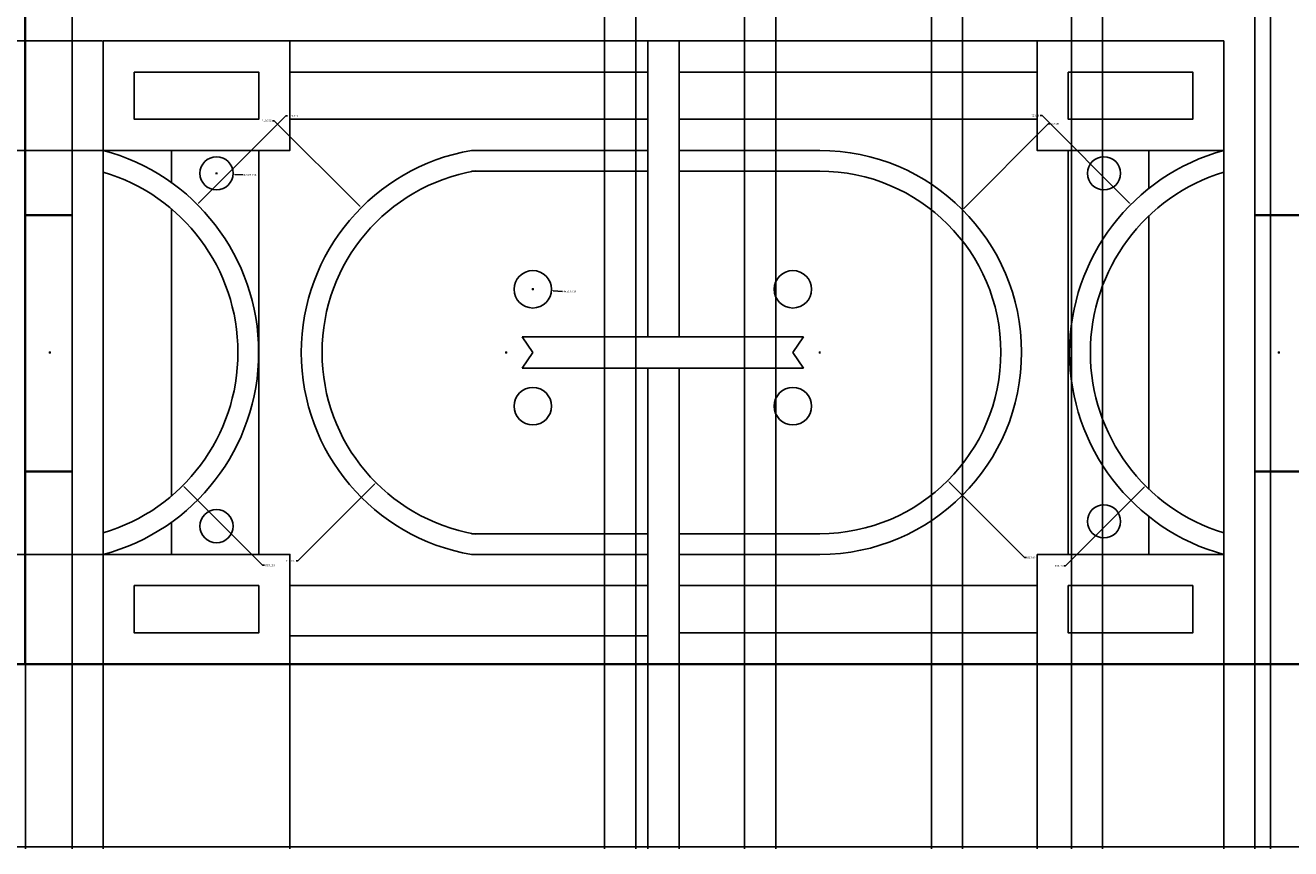
# Model space of a CAD drawing. Units: inches. Extents: x 2612 to 2948, y 481 to 865.
# Tile 2 of 7: x 2708 to 2830, y 481 to 561. Entities that reach past the tile are written whole.
import ezdxf

# ---------------------------------------------------------------- set-up
doc = ezdxf.new("R2010")
doc.units = ezdxf.units.IN
for name, color, linetype, lineweight in [('A-ANNO-DIMS', 2, 'Continuous', 18), ('A-DOOR', 4, 'Continuous', 25), ('A-ELEV', 7, 'Continuous', 35)]:
    doc.layers.add(name, color=color, linetype=linetype, lineweight=lineweight)
doc.styles.get("Standard").update_dxf_attribs({"font": 'arial.ttf'})
doc.dimstyles.get("Standard").update_dxf_attribs({"dimtxt": 0.18, "dimasz": 0.18, "dimexe": 0.18, "dimexo": 0.0625, "dimgap": 0.09, "dimtad": 0, "dimtih": 1, "dimtoh": 1, "dimdec": 4, "dimzin": 0, "dimdsep": 46, "dimtxsty": 'Standard', "dimcen": 0.09, "dimadec": 0, "dimazin": 0, "dimtfac": 1, "dimtdec": 4, "dimtofl": 0, "dimtmove": 0, "dimatfit": 3, "dimfxl": 1, "dimtolj": 1, "dimtzin": 0, "dimarcsym": 0})

# ---------------------------------------------------------------- blocks, each defined once
blk = doc.blocks.new('*D22')
at = {"layer": 'A-ANNO-DIMS', "color": 0, "lineweight": -2, "transparency": 16777216}
for p, q in [((2708.31, 648.98), (2708.31, 481.26)), ((2831.31, 570.98), (2831.31, 481.26)), ((2708.49, 481.44), (2769.53, 481.44)), ((2831.13, 481.44), (2770.09, 481.44))]:
    blk.add_line(p, q, dxfattribs=at)
at = {"layer": 'A-ANNO-DIMS', "color": 0, "transparency": 16777216}
for points in [[(2708.49, 481.47), (2708.49, 481.41), (2708.31, 481.44)], [(2831.13, 481.47), (2831.13, 481.41), (2831.31, 481.44)]]:
    blk.add_solid(points, dxfattribs=at)
at = {"layer": 'Defpoints', "color": 0, "transparency": 16777216}
for p in [(2708.31, 649.04), (2831.31, 571.04), (2831.31, 481.44)]:
    blk.add_point(p, dxfattribs=at)
at = {"layer": 'A-ANNO-DIMS', "color": 0, "transparency": 16777216, "insert": (2769.81, 481.44), "char_height": 0.18, "attachment_point": 5}
blk.add_mtext('\\A1;123', dxfattribs=at)
blk = doc.blocks.new('*D52')
at = {"layer": 'A-ANNO-DIMS', "color": 0, "lineweight": -2, "transparency": 16777216}
for p, q in [((2712.81, 498.98), (2712.81, 481.26)), ((2715.81, 498.98), (2715.81, 481.26)), ((2712.99, 481.44), (2714.16, 481.44)), ((2715.63, 481.44), (2714.46, 481.44))]:
    blk.add_line(p, q, dxfattribs=at)
at = {"layer": 'A-ANNO-DIMS', "color": 0, "transparency": 16777216}
for points in [[(2712.99, 481.47), (2712.99, 481.41), (2712.81, 481.44)], [(2715.63, 481.47), (2715.63, 481.41), (2715.81, 481.44)]]:
    blk.add_solid(points, dxfattribs=at)
at = {"layer": 'Defpoints', "color": 0, "transparency": 16777216}
for p in [(2712.81, 499.04), (2715.81, 499.04), (2715.81, 481.44)]:
    blk.add_point(p, dxfattribs=at)
at = {"layer": 'A-ANNO-DIMS', "color": 0, "transparency": 16777216, "insert": (2714.31, 481.44), "char_height": 0.18, "attachment_point": 5}
blk.add_mtext('\\A1;3', dxfattribs=at)
blk = doc.blocks.new('*D53')
at = {"layer": 'A-ANNO-DIMS', "color": 0, "lineweight": -2, "transparency": 16777216}
for p, q in [((2715.81, 498.98), (2715.81, 481.26)), ((2733.81, 498.98), (2733.81, 481.26)), ((2715.99, 481.44), (2724.6, 481.44)), ((2733.63, 481.44), (2725.02, 481.44))]:
    blk.add_line(p, q, dxfattribs=at)
at = {"layer": 'A-ANNO-DIMS', "color": 0, "transparency": 16777216}
for points in [[(2715.99, 481.47), (2715.99, 481.41), (2715.81, 481.44)], [(2733.63, 481.47), (2733.63, 481.41), (2733.81, 481.44)]]:
    blk.add_solid(points, dxfattribs=at)
at = {"layer": 'Defpoints', "color": 0, "transparency": 16777216}
for p in [(2715.81, 499.04), (2733.81, 499.04), (2733.81, 481.44)]:
    blk.add_point(p, dxfattribs=at)
at = {"layer": 'A-ANNO-DIMS', "color": 0, "transparency": 16777216, "insert": (2724.81, 481.44), "char_height": 0.18, "attachment_point": 5}
blk.add_mtext('\\A1;18', dxfattribs=at)
blk = doc.blocks.new('*D54')
at = {"layer": 'A-ANNO-DIMS', "color": 0, "lineweight": -2, "transparency": 16777216}
for p, q in [((2733.81, 498.98), (2733.81, 481.26)), ((2768.31, 498.98), (2768.31, 481.26)), ((2733.99, 481.44), (2750.73, 481.44)), ((2768.13, 481.44), (2751.38, 481.44))]:
    blk.add_line(p, q, dxfattribs=at)
at = {"layer": 'A-ANNO-DIMS', "color": 0, "transparency": 16777216}
for points in [[(2733.99, 481.47), (2733.99, 481.41), (2733.81, 481.44)], [(2768.13, 481.47), (2768.13, 481.41), (2768.31, 481.44)]]:
    blk.add_solid(points, dxfattribs=at)
at = {"layer": 'Defpoints', "color": 0, "transparency": 16777216}
for p in [(2733.81, 499.04), (2768.31, 499.04), (2768.31, 481.44)]:
    blk.add_point(p, dxfattribs=at)
at = {"layer": 'A-ANNO-DIMS', "color": 0, "transparency": 16777216, "insert": (2751.06, 481.44), "char_height": 0.18, "attachment_point": 5}
blk.add_mtext('\\A1;34.5', dxfattribs=at)
blk = doc.blocks.new('*D55')
at = {"layer": 'A-ANNO-DIMS', "color": 0, "lineweight": -2, "transparency": 16777216}
for p, q in [((2768.31, 498.98), (2768.31, 481.26)), ((2771.31, 498.98), (2771.31, 481.26)), ((2768.49, 481.44), (2769.66, 481.44)), ((2771.13, 481.44), (2769.96, 481.44))]:
    blk.add_line(p, q, dxfattribs=at)
at = {"layer": 'A-ANNO-DIMS', "color": 0, "transparency": 16777216}
for points in [[(2768.49, 481.47), (2768.49, 481.41), (2768.31, 481.44)], [(2771.13, 481.47), (2771.13, 481.41), (2771.31, 481.44)]]:
    blk.add_solid(points, dxfattribs=at)
at = {"layer": 'Defpoints', "color": 0, "transparency": 16777216}
for p in [(2768.31, 499.04), (2771.31, 499.04), (2771.31, 481.44)]:
    blk.add_point(p, dxfattribs=at)
at = {"layer": 'A-ANNO-DIMS', "color": 0, "transparency": 16777216, "insert": (2769.81, 481.44), "char_height": 0.18, "attachment_point": 5}
blk.add_mtext('\\A1;3', dxfattribs=at)
blk = doc.blocks.new('*D56')
at = {"layer": 'A-ANNO-DIMS', "color": 0, "lineweight": -2, "transparency": 16777216}
for p, q in [((2771.31, 498.98), (2771.31, 481.26)), ((2805.81, 498.98), (2805.81, 481.26)), ((2771.49, 481.44), (2788.23, 481.44)), ((2805.63, 481.44), (2788.88, 481.44))]:
    blk.add_line(p, q, dxfattribs=at)
at = {"layer": 'A-ANNO-DIMS', "color": 0, "transparency": 16777216}
for points in [[(2771.49, 481.47), (2771.49, 481.41), (2771.31, 481.44)], [(2805.63, 481.47), (2805.63, 481.41), (2805.81, 481.44)]]:
    blk.add_solid(points, dxfattribs=at)
at = {"layer": 'Defpoints', "color": 0, "transparency": 16777216}
for p in [(2771.31, 499.04), (2805.81, 499.04), (2805.81, 481.44)]:
    blk.add_point(p, dxfattribs=at)
at = {"layer": 'A-ANNO-DIMS', "color": 0, "transparency": 16777216, "insert": (2788.56, 481.44), "char_height": 0.18, "attachment_point": 5}
blk.add_mtext('\\A1;34.5', dxfattribs=at)
blk = doc.blocks.new('*D57')
at = {"layer": 'A-ANNO-DIMS', "color": 0, "lineweight": -2, "transparency": 16777216}
for p, q in [((2805.81, 498.98), (2805.81, 481.26)), ((2823.81, 498.98), (2823.81, 481.26)), ((2805.99, 481.44), (2814.6, 481.44)), ((2823.63, 481.44), (2815.02, 481.44))]:
    blk.add_line(p, q, dxfattribs=at)
at = {"layer": 'A-ANNO-DIMS', "color": 0, "transparency": 16777216}
for points in [[(2805.99, 481.47), (2805.99, 481.41), (2805.81, 481.44)], [(2823.63, 481.47), (2823.63, 481.41), (2823.81, 481.44)]]:
    blk.add_solid(points, dxfattribs=at)
at = {"layer": 'Defpoints', "color": 0, "transparency": 16777216}
for p in [(2805.81, 499.04), (2823.81, 499.04), (2823.81, 481.44)]:
    blk.add_point(p, dxfattribs=at)
at = {"layer": 'A-ANNO-DIMS', "color": 0, "transparency": 16777216, "insert": (2814.81, 481.44), "char_height": 0.18, "attachment_point": 5}
blk.add_mtext('\\A1;18', dxfattribs=at)
blk = doc.blocks.new('*D58')
at = {"layer": 'A-ANNO-DIMS', "color": 0, "lineweight": -2, "transparency": 16777216}
for p, q in [((2823.81, 498.98), (2823.81, 481.26)), ((2826.81, 498.98), (2826.81, 481.26)), ((2823.99, 481.44), (2825.16, 481.44)), ((2826.63, 481.44), (2825.46, 481.44))]:
    blk.add_line(p, q, dxfattribs=at)
at = {"layer": 'A-ANNO-DIMS', "color": 0, "transparency": 16777216}
for points in [[(2823.99, 481.47), (2823.99, 481.41), (2823.81, 481.44)], [(2826.63, 481.47), (2826.63, 481.41), (2826.81, 481.44)]]:
    blk.add_solid(points, dxfattribs=at)
at = {"layer": 'Defpoints', "color": 0, "transparency": 16777216}
for p in [(2823.81, 499.04), (2826.81, 499.04), (2826.81, 481.44)]:
    blk.add_point(p, dxfattribs=at)
at = {"layer": 'A-ANNO-DIMS', "color": 0, "transparency": 16777216, "insert": (2825.31, 481.44), "char_height": 0.18, "attachment_point": 5}
blk.add_mtext('\\A1;3', dxfattribs=at)
blk = doc.blocks.new('*D59')
at = {"layer": 'A-ANNO-DIMS', "color": 0, "lineweight": -2, "transparency": 16777216}
for p, q in [((2715.74, 509.59), (2612.53, 509.59)), ((2612.71, 509.41), (2612.71, 504.5)), ((2612.71, 499.22), (2612.71, 504.14)), ((2715.74, 499.04), (2612.53, 499.04))]:
    blk.add_line(p, q, dxfattribs=at)
at = {"layer": 'A-ANNO-DIMS', "color": 0, "transparency": 16777216}
for points in [[(2612.68, 509.41), (2612.74, 509.41), (2612.71, 509.59)], [(2612.68, 499.22), (2612.74, 499.22), (2612.71, 499.04)]]:
    blk.add_solid(points, dxfattribs=at)
at = {"layer": 'Defpoints', "color": 0, "transparency": 16777216}
for p in [(2612.71, 509.59), (2715.81, 509.59), (2715.81, 499.04)]:
    blk.add_point(p, dxfattribs=at)
at = {"layer": 'A-ANNO-DIMS', "color": 0, "transparency": 16777216, "insert": (2612.71, 504.32), "char_height": 0.18, "attachment_point": 5}
blk.add_mtext('\\A1;10.548', dxfattribs=at)
blk = doc.blocks.new('*D60')
at = {"layer": 'A-ANNO-DIMS', "color": 0, "lineweight": -2, "transparency": 16777216}
for p, q in [((2715.74, 548.5), (2612.53, 548.5)), ((2612.71, 548.32), (2612.71, 529.23)), ((2612.71, 509.77), (2612.71, 528.86)), ((2715.74, 509.59), (2612.53, 509.59))]:
    blk.add_line(p, q, dxfattribs=at)
at = {"layer": 'A-ANNO-DIMS', "color": 0, "transparency": 16777216}
for points in [[(2612.68, 548.32), (2612.74, 548.32), (2612.71, 548.5)], [(2612.68, 509.77), (2612.74, 509.77), (2612.71, 509.59)]]:
    blk.add_solid(points, dxfattribs=at)
at = {"layer": 'Defpoints', "color": 0, "transparency": 16777216}
for p in [(2612.71, 548.5), (2715.81, 548.5), (2715.81, 509.59)]:
    blk.add_point(p, dxfattribs=at)
at = {"layer": 'A-ANNO-DIMS', "color": 0, "transparency": 16777216, "insert": (2612.71, 529.04), "char_height": 0.18, "attachment_point": 5}
blk.add_mtext('\\A1;38.9', dxfattribs=at)
blk = doc.blocks.new('*D61')
at = {"layer": 'A-ANNO-DIMS', "color": 0, "lineweight": -2, "transparency": 16777216}
for p, q in [((2715.74, 559.04), (2612.53, 559.04)), ((2612.71, 558.86), (2612.71, 553.95)), ((2612.71, 548.68), (2612.71, 553.59)), ((2715.74, 548.5), (2612.53, 548.5))]:
    blk.add_line(p, q, dxfattribs=at)
at = {"layer": 'A-ANNO-DIMS', "color": 0, "transparency": 16777216}
for points in [[(2612.68, 558.86), (2612.74, 558.86), (2612.71, 559.04)], [(2612.68, 548.68), (2612.74, 548.68), (2612.71, 548.5)]]:
    blk.add_solid(points, dxfattribs=at)
at = {"layer": 'Defpoints', "color": 0, "transparency": 16777216}
for p in [(2612.71, 559.04), (2715.81, 559.04), (2715.81, 548.5)]:
    blk.add_point(p, dxfattribs=at)
at = {"layer": 'A-ANNO-DIMS', "color": 0, "transparency": 16777216, "insert": (2612.71, 553.77), "char_height": 0.18, "attachment_point": 5}
blk.add_mtext('\\A1;10.548', dxfattribs=at)
blk = doc.blocks.new('*D62')
at = {"layer": 'A-ANNO-DIMS', "color": 0, "lineweight": -2, "transparency": 16777216}
for p, q in [((2712.74, 562.04), (2612.53, 562.04)), ((2612.71, 561.86), (2612.71, 560.73)), ((2612.71, 559.22), (2612.71, 560.36)), ((2715.74, 559.04), (2612.53, 559.04))]:
    blk.add_line(p, q, dxfattribs=at)
at = {"layer": 'A-ANNO-DIMS', "color": 0, "transparency": 16777216}
for points in [[(2612.68, 561.86), (2612.74, 561.86), (2612.71, 562.04)], [(2612.68, 559.22), (2612.74, 559.22), (2612.71, 559.04)]]:
    blk.add_solid(points, dxfattribs=at)
at = {"layer": 'Defpoints', "color": 0, "transparency": 16777216}
for p in [(2612.71, 562.04), (2712.81, 562.04), (2715.81, 559.04)]:
    blk.add_point(p, dxfattribs=at)
at = {"layer": 'A-ANNO-DIMS', "color": 0, "transparency": 16777216, "insert": (2612.71, 560.54), "char_height": 0.18, "attachment_point": 5}
blk.add_mtext('\\A1;3', dxfattribs=at)
blk = doc.blocks.new('*D64')
at = {"layer": 'A-ANNO-DIMS', "color": 0, "lineweight": -2, "transparency": 16777216}
for p, q in [((2826.87, 562.04), (2948.09, 562.04)), ((2947.91, 561.86), (2947.91, 530.73)), ((2947.91, 499.22), (2947.91, 530.36)), ((2826.87, 499.04), (2948.09, 499.04))]:
    blk.add_line(p, q, dxfattribs=at)
at = {"layer": 'A-ANNO-DIMS', "color": 0, "transparency": 16777216}
for points in [[(2947.88, 561.86), (2947.94, 561.86), (2947.91, 562.04)], [(2947.88, 499.22), (2947.94, 499.22), (2947.91, 499.04)]]:
    blk.add_solid(points, dxfattribs=at)
at = {"layer": 'Defpoints', "color": 0, "transparency": 16777216}
for p in [(2826.81, 562.04), (2947.91, 562.04), (2826.81, 499.04)]:
    blk.add_point(p, dxfattribs=at)
at = {"layer": 'A-ANNO-DIMS', "color": 0, "transparency": 16777216, "insert": (2947.91, 530.54), "char_height": 0.18, "attachment_point": 5}
blk.add_mtext('\\A1;63', dxfattribs=at)
blk = doc.blocks.new('*D66')
at = {"layer": 'A-ANNO-DIMS', "color": 0, "lineweight": -2, "transparency": 16777216}
for p, q in [((2767.13, 711.98), (2767.13, 481.26)), ((2764.13, 708.98), (2764.13, 481.26)), ((2764.31, 481.44), (2765.48, 481.44)), ((2766.95, 481.44), (2765.78, 481.44))]:
    blk.add_line(p, q, dxfattribs=at)
at = {"layer": 'A-ANNO-DIMS', "color": 0, "transparency": 16777216}
for points in [[(2764.31, 481.47), (2764.31, 481.41), (2764.13, 481.44)], [(2766.95, 481.47), (2766.95, 481.41), (2767.13, 481.44)]]:
    blk.add_solid(points, dxfattribs=at)
at = {"layer": 'Defpoints', "color": 0, "transparency": 16777216}
for p in [(2767.13, 712.04), (2764.13, 709.04), (2767.13, 481.44)]:
    blk.add_point(p, dxfattribs=at)
at = {"layer": 'A-ANNO-DIMS', "color": 0, "transparency": 16777216, "insert": (2765.63, 481.44), "char_height": 0.18, "attachment_point": 5}
blk.add_mtext('\\A1;3', dxfattribs=at)
blk = doc.blocks.new('*D67')
at = {"layer": 'A-ANNO-DIMS', "color": 0, "lineweight": -2, "transparency": 16777216}
for p, q in [((2767.13, 711.98), (2767.13, 481.26)), ((2777.63, 711.98), (2777.63, 481.26)), ((2767.31, 481.44), (2772.06, 481.44)), ((2777.45, 481.44), (2772.7, 481.44))]:
    blk.add_line(p, q, dxfattribs=at)
at = {"layer": 'A-ANNO-DIMS', "color": 0, "transparency": 16777216}
for points in [[(2767.31, 481.47), (2767.31, 481.41), (2767.13, 481.44)], [(2777.45, 481.47), (2777.45, 481.41), (2777.63, 481.44)]]:
    blk.add_solid(points, dxfattribs=at)
at = {"layer": 'Defpoints', "color": 0, "transparency": 16777216}
for p in [(2767.13, 712.04), (2777.63, 712.04), (2777.63, 481.44)]:
    blk.add_point(p, dxfattribs=at)
at = {"layer": 'A-ANNO-DIMS', "color": 0, "transparency": 16777216, "insert": (2772.38, 481.44), "char_height": 0.18, "attachment_point": 5}
blk.add_mtext('\\A1;10.5', dxfattribs=at)
blk = doc.blocks.new('*D68')
at = {"layer": 'A-ANNO-DIMS', "color": 0, "lineweight": -2, "transparency": 16777216}
for p, q in [((2777.63, 711.98), (2777.63, 481.26)), ((2780.63, 711.98), (2780.63, 481.26)), ((2777.81, 481.44), (2778.98, 481.44)), ((2780.45, 481.44), (2779.28, 481.44))]:
    blk.add_line(p, q, dxfattribs=at)
at = {"layer": 'A-ANNO-DIMS', "color": 0, "transparency": 16777216}
for points in [[(2777.81, 481.47), (2777.81, 481.41), (2777.63, 481.44)], [(2780.45, 481.47), (2780.45, 481.41), (2780.63, 481.44)]]:
    blk.add_solid(points, dxfattribs=at)
at = {"layer": 'Defpoints', "color": 0, "transparency": 16777216}
for p in [(2777.63, 712.04), (2780.63, 712.04), (2780.63, 481.44)]:
    blk.add_point(p, dxfattribs=at)
at = {"layer": 'A-ANNO-DIMS', "color": 0, "transparency": 16777216, "insert": (2779.13, 481.44), "char_height": 0.18, "attachment_point": 5}
blk.add_mtext('\\A1;3', dxfattribs=at)
blk = doc.blocks.new('*D69')
at = {"layer": 'A-ANNO-DIMS', "color": 0, "lineweight": -2, "transparency": 16777216}
for p, q in [((2780.63, 711.98), (2780.63, 481.26)), ((2795.63, 711.98), (2795.63, 481.26)), ((2780.81, 481.44), (2787.92, 481.44)), ((2795.45, 481.44), (2788.34, 481.44))]:
    blk.add_line(p, q, dxfattribs=at)
at = {"layer": 'A-ANNO-DIMS', "color": 0, "transparency": 16777216}
for points in [[(2780.81, 481.47), (2780.81, 481.41), (2780.63, 481.44)], [(2795.45, 481.47), (2795.45, 481.41), (2795.63, 481.44)]]:
    blk.add_solid(points, dxfattribs=at)
at = {"layer": 'Defpoints', "color": 0, "transparency": 16777216}
for p in [(2780.63, 712.04), (2795.63, 712.04), (2795.63, 481.44)]:
    blk.add_point(p, dxfattribs=at)
at = {"layer": 'A-ANNO-DIMS', "color": 0, "transparency": 16777216, "insert": (2788.13, 481.44), "char_height": 0.18, "attachment_point": 5}
blk.add_mtext('\\A1;15', dxfattribs=at)
blk = doc.blocks.new('*D70')
at = {"layer": 'A-ANNO-DIMS', "color": 0, "lineweight": -2, "transparency": 16777216}
for p, q in [((2795.63, 711.98), (2795.63, 481.26)), ((2798.63, 711.98), (2798.63, 481.26)), ((2795.81, 481.44), (2796.98, 481.44)), ((2798.45, 481.44), (2797.28, 481.44))]:
    blk.add_line(p, q, dxfattribs=at)
at = {"layer": 'A-ANNO-DIMS', "color": 0, "transparency": 16777216}
for points in [[(2795.81, 481.47), (2795.81, 481.41), (2795.63, 481.44)], [(2798.45, 481.47), (2798.45, 481.41), (2798.63, 481.44)]]:
    blk.add_solid(points, dxfattribs=at)
at = {"layer": 'Defpoints', "color": 0, "transparency": 16777216}
for p in [(2795.63, 712.04), (2798.63, 712.04), (2798.63, 481.44)]:
    blk.add_point(p, dxfattribs=at)
at = {"layer": 'A-ANNO-DIMS', "color": 0, "transparency": 16777216, "insert": (2797.13, 481.44), "char_height": 0.18, "attachment_point": 5}
blk.add_mtext('\\A1;3', dxfattribs=at)
blk = doc.blocks.new('*D71')
at = {"layer": 'A-ANNO-DIMS', "color": 0, "lineweight": -2, "transparency": 16777216}
for p, q in [((2798.63, 711.98), (2798.63, 481.26)), ((2809.13, 711.98), (2809.13, 481.26)), ((2798.81, 481.44), (2803.56, 481.44)), ((2808.95, 481.44), (2804.2, 481.44))]:
    blk.add_line(p, q, dxfattribs=at)
at = {"layer": 'A-ANNO-DIMS', "color": 0, "transparency": 16777216}
for points in [[(2798.81, 481.47), (2798.81, 481.41), (2798.63, 481.44)], [(2808.95, 481.47), (2808.95, 481.41), (2809.13, 481.44)]]:
    blk.add_solid(points, dxfattribs=at)
at = {"layer": 'Defpoints', "color": 0, "transparency": 16777216}
for p in [(2798.63, 712.04), (2809.13, 712.04), (2809.13, 481.44)]:
    blk.add_point(p, dxfattribs=at)
at = {"layer": 'A-ANNO-DIMS', "color": 0, "transparency": 16777216, "insert": (2803.88, 481.44), "char_height": 0.18, "attachment_point": 5}
blk.add_mtext('\\A1;10.5', dxfattribs=at)
blk = doc.blocks.new('*D72')
at = {"layer": 'A-ANNO-DIMS', "color": 0, "lineweight": -2, "transparency": 16777216}
for p, q in [((2809.13, 711.98), (2809.13, 481.26)), ((2812.13, 708.98), (2812.13, 481.26)), ((2809.31, 481.44), (2810.48, 481.44)), ((2811.95, 481.44), (2810.78, 481.44))]:
    blk.add_line(p, q, dxfattribs=at)
at = {"layer": 'A-ANNO-DIMS', "color": 0, "transparency": 16777216}
for points in [[(2809.31, 481.47), (2809.31, 481.41), (2809.13, 481.44)], [(2811.95, 481.47), (2811.95, 481.41), (2812.13, 481.44)]]:
    blk.add_solid(points, dxfattribs=at)
at = {"layer": 'Defpoints', "color": 0, "transparency": 16777216}
for p in [(2809.13, 712.04), (2812.13, 709.04), (2812.13, 481.44)]:
    blk.add_point(p, dxfattribs=at)
at = {"layer": 'A-ANNO-DIMS', "color": 0, "transparency": 16777216, "insert": (2810.63, 481.44), "char_height": 0.18, "attachment_point": 5}
blk.add_mtext('\\A1;3', dxfattribs=at)
blk = doc.blocks.new('*D73')
at = {"layer": 'A-ANNO-DIMS', "color": 0, "lineweight": -2, "transparency": 16777216}
for p, q in [((2812.13, 708.98), (2812.13, 481.26)), ((2828.31, 708.98), (2828.31, 481.26)), ((2812.31, 481.44), (2819.76, 481.44)), ((2828.13, 481.44), (2820.67, 481.44))]:
    blk.add_line(p, q, dxfattribs=at)
at = {"layer": 'A-ANNO-DIMS', "color": 0, "transparency": 16777216}
for points in [[(2812.31, 481.47), (2812.31, 481.41), (2812.13, 481.44)], [(2828.13, 481.47), (2828.13, 481.41), (2828.31, 481.44)]]:
    blk.add_solid(points, dxfattribs=at)
at = {"layer": 'Defpoints', "color": 0, "transparency": 16777216}
for p in [(2812.13, 709.04), (2828.31, 709.04), (2828.31, 481.44)]:
    blk.add_point(p, dxfattribs=at)
at = {"layer": 'A-ANNO-DIMS', "color": 0, "transparency": 16777216, "insert": (2820.22, 481.44), "char_height": 0.18, "attachment_point": 5}
blk.add_mtext('\\A1;16.177', dxfattribs=at)
blk = doc.blocks.new('*D74')
at = {"layer": 'A-ANNO-DIMS', "color": 0, "lineweight": -2, "transparency": 16777216}
for p, q in [((2831.31, 711.98), (2831.31, 481.26)), ((2828.31, 708.98), (2828.31, 481.26)), ((2828.49, 481.44), (2829.66, 481.44)), ((2831.13, 481.44), (2829.96, 481.44))]:
    blk.add_line(p, q, dxfattribs=at)
at = {"layer": 'A-ANNO-DIMS', "color": 0, "transparency": 16777216}
for points in [[(2828.49, 481.47), (2828.49, 481.41), (2828.31, 481.44)], [(2831.13, 481.47), (2831.13, 481.41), (2831.31, 481.44)]]:
    blk.add_solid(points, dxfattribs=at)
at = {"layer": 'Defpoints', "color": 0, "transparency": 16777216}
for p in [(2831.31, 712.04), (2828.31, 709.04), (2831.31, 481.44)]:
    blk.add_point(p, dxfattribs=at)
at = {"layer": 'A-ANNO-DIMS', "color": 0, "transparency": 16777216, "insert": (2829.81, 481.44), "char_height": 0.18, "attachment_point": 5}
blk.add_mtext('\\A1;3', dxfattribs=at)
blk = doc.blocks.new('*D87')
at = {"layer": 'A-ANNO-DIMS', "color": 0, "lineweight": -2, "transparency": 16777216}
for p, q in [((2630.31, 498.98), (2630.31, 481.26)), ((2930.31, 498.98), (2930.31, 481.26)), ((2630.49, 481.44), (2780.02, 481.44)), ((2930.13, 481.44), (2780.6, 481.44))]:
    blk.add_line(p, q, dxfattribs=at)
at = {"layer": 'A-ANNO-DIMS', "color": 0, "transparency": 16777216}
for points in [[(2630.49, 481.47), (2630.49, 481.41), (2630.31, 481.44)], [(2930.13, 481.47), (2930.13, 481.41), (2930.31, 481.44)]]:
    blk.add_solid(points, dxfattribs=at)
at = {"layer": 'Defpoints', "color": 0, "transparency": 16777216}
for p in [(2630.31, 499.04), (2930.31, 499.04), (2930.31, 481.44)]:
    blk.add_point(p, dxfattribs=at)
at = {"layer": 'A-ANNO-DIMS', "color": 0, "transparency": 16777216, "insert": (2780.31, 481.44), "char_height": 0.18, "attachment_point": 5}
blk.add_mtext('\\A1;300', dxfattribs=at)
blk = doc.blocks.new('*D95')
at = {"layer": 'A-ANNO-DIMS', "color": 0, "lineweight": -2, "transparency": 16777216}
for p, q in [((2733.41, 551.83), (2725.01, 543.41)), ((2733.59, 551.83), (2733.41, 551.83)), ((2710.59, 529.04), (2710.77, 529.04)), ((2710.68, 528.95), (2710.68, 529.13))]:
    blk.add_line(p, q, dxfattribs=at)
at = {"layer": 'A-ANNO-DIMS', "color": 0, "transparency": 16777216}
blk.add_solid([(2724.99, 543.43), (2725.03, 543.39), (2724.89, 543.29)], dxfattribs=at)
at = {"layer": 'Defpoints', "color": 0, "transparency": 16777216}
for p in [(2724.89, 543.29), (2710.68, 529.04)]:
    blk.add_point(p, dxfattribs=at)
at = {"layer": 'A-ANNO-DIMS', "color": 0, "transparency": 16777216, "insert": (2734.14, 551.83), "char_height": 0.18, "attachment_point": 5}
blk.add_mtext('\\A1;R20.116', dxfattribs=at)
blk = doc.blocks.new('*D96')
at = {"layer": 'A-ANNO-DIMS', "color": 0, "lineweight": -2, "transparency": 16777216}
for p, q in [((2710.59, 529.04), (2710.77, 529.04)), ((2710.68, 528.95), (2710.68, 529.13)), ((2731.17, 508.55), (2723.61, 516.11)), ((2731.35, 508.55), (2731.17, 508.55))]:
    blk.add_line(p, q, dxfattribs=at)
at = {"layer": 'A-ANNO-DIMS', "color": 0, "transparency": 16777216}
blk.add_solid([(2723.64, 516.13), (2723.59, 516.08), (2723.49, 516.23)], dxfattribs=at)
at = {"layer": 'Defpoints', "color": 0, "transparency": 16777216}
for p in [(2710.68, 529.04), (2723.49, 516.23)]:
    blk.add_point(p, dxfattribs=at)
at = {"layer": 'A-ANNO-DIMS', "color": 0, "transparency": 16777216, "insert": (2731.9, 508.55), "char_height": 0.18, "attachment_point": 5}
blk.add_mtext('\\A1;R18.116', dxfattribs=at)
blk = doc.blocks.new('*D97')
at = {"layer": 'A-ANNO-DIMS', "color": 0, "lineweight": -2, "transparency": 16777216}
for p, q in [((2732.12, 551.36), (2732.3, 551.36)), ((2732.3, 551.36), (2740.55, 543.12)), ((2754.55, 529.04), (2754.73, 529.04)), ((2754.64, 528.95), (2754.64, 529.13))]:
    blk.add_line(p, q, dxfattribs=at)
at = {"layer": 'A-ANNO-DIMS', "color": 0, "transparency": 16777216}
blk.add_solid([(2740.57, 543.14), (2740.53, 543.1), (2740.68, 542.99)], dxfattribs=at)
at = {"layer": 'Defpoints', "color": 0, "transparency": 16777216}
for p in [(2740.68, 542.99), (2754.64, 529.04)]:
    blk.add_point(p, dxfattribs=at)
at = {"layer": 'A-ANNO-DIMS', "color": 0, "transparency": 16777216, "insert": (2731.57, 551.36), "char_height": 0.18, "attachment_point": 5}
blk.add_mtext('\\A1;R19.735', dxfattribs=at)
blk = doc.blocks.new('*D98')
at = {"layer": 'A-ANNO-DIMS', "color": 0, "lineweight": -2, "transparency": 16777216}
for p, q in [((2754.55, 529.04), (2754.73, 529.04)), ((2754.64, 528.95), (2754.64, 529.13)), ((2734.58, 508.98), (2741.97, 516.37)), ((2734.4, 508.98), (2734.58, 508.98))]:
    blk.add_line(p, q, dxfattribs=at)
at = {"layer": 'A-ANNO-DIMS', "color": 0, "transparency": 16777216}
blk.add_solid([(2741.95, 516.4), (2742, 516.35), (2742.1, 516.5)], dxfattribs=at)
at = {"layer": 'Defpoints', "color": 0, "transparency": 16777216}
for p in [(2754.64, 529.04), (2742.1, 516.5)]:
    blk.add_point(p, dxfattribs=at)
at = {"layer": 'A-ANNO-DIMS', "color": 0, "transparency": 16777216, "insert": (2733.85, 508.98), "char_height": 0.18, "attachment_point": 5}
blk.add_mtext('\\A1;R17.735', dxfattribs=at)
blk = doc.blocks.new('*D99')
at = {"layer": 'A-ANNO-DIMS', "color": 0, "lineweight": -2, "transparency": 16777216}
for p, q in [((2806.87, 551.05), (2798.74, 542.92)), ((2807.05, 551.05), (2806.87, 551.05)), ((2784.77, 529.04), (2784.95, 529.04)), ((2784.86, 528.95), (2784.86, 529.13))]:
    blk.add_line(p, q, dxfattribs=at)
at = {"layer": 'A-ANNO-DIMS', "color": 0, "transparency": 16777216}
blk.add_solid([(2798.72, 542.95), (2798.77, 542.9), (2798.62, 542.8)], dxfattribs=at)
at = {"layer": 'Defpoints', "color": 0, "transparency": 16777216}
for p in [(2798.62, 542.8), (2784.86, 529.04)]:
    blk.add_point(p, dxfattribs=at)
at = {"layer": 'A-ANNO-DIMS', "color": 0, "transparency": 16777216, "insert": (2807.53, 551.05), "char_height": 0.18, "attachment_point": 5}
blk.add_mtext('\\A1;R19.45', dxfattribs=at)
blk = doc.blocks.new('*D100')
at = {"layer": 'A-ANNO-DIMS', "color": 0, "lineweight": -2, "transparency": 16777216}
for p, q in [((2784.77, 529.04), (2784.95, 529.04)), ((2784.86, 528.95), (2784.86, 529.13)), ((2804.6, 509.29), (2797.33, 516.57)), ((2804.78, 509.29), (2804.6, 509.29))]:
    blk.add_line(p, q, dxfattribs=at)
at = {"layer": 'A-ANNO-DIMS', "color": 0, "transparency": 16777216}
blk.add_solid([(2797.35, 516.59), (2797.31, 516.55), (2797.2, 516.7)], dxfattribs=at)
at = {"layer": 'Defpoints', "color": 0, "transparency": 16777216}
for p in [(2784.86, 529.04), (2797.2, 516.7)]:
    blk.add_point(p, dxfattribs=at)
at = {"layer": 'A-ANNO-DIMS', "color": 0, "transparency": 16777216, "insert": (2805.26, 509.29), "char_height": 0.18, "attachment_point": 5}
blk.add_mtext('\\A1;R17.45', dxfattribs=at)
blk = doc.blocks.new('*D101')
at = {"layer": 'A-ANNO-DIMS', "color": 0, "lineweight": -2, "transparency": 16777216}
for p, q in [((2806.12, 551.85), (2806.3, 551.85)), ((2806.3, 551.85), (2814.72, 543.43)), ((2829.01, 529.04), (2829.19, 529.04)), ((2829.1, 528.95), (2829.1, 529.13))]:
    blk.add_line(p, q, dxfattribs=at)
at = {"layer": 'A-ANNO-DIMS', "color": 0, "transparency": 16777216}
blk.add_solid([(2814.74, 543.45), (2814.7, 543.41), (2814.85, 543.3)], dxfattribs=at)
at = {"layer": 'Defpoints', "color": 0, "transparency": 16777216}
for p in [(2814.85, 543.3), (2829.1, 529.04)]:
    blk.add_point(p, dxfattribs=at)
at = {"layer": 'A-ANNO-DIMS', "color": 0, "transparency": 16777216, "insert": (2805.64, 551.85), "char_height": 0.18, "attachment_point": 5}
blk.add_mtext('\\A1;R20.16', dxfattribs=at)
blk = doc.blocks.new('*D102')
at = {"layer": 'A-ANNO-DIMS', "color": 0, "lineweight": -2, "transparency": 16777216}
for p, q in [((2829.01, 529.04), (2829.19, 529.04)), ((2829.1, 528.95), (2829.1, 529.13)), ((2808.56, 508.5), (2816.14, 516.08)), ((2808.38, 508.5), (2808.56, 508.5))]:
    blk.add_line(p, q, dxfattribs=at)
at = {"layer": 'A-ANNO-DIMS', "color": 0, "transparency": 16777216}
blk.add_solid([(2816.11, 516.1), (2816.16, 516.05), (2816.26, 516.2)], dxfattribs=at)
at = {"layer": 'Defpoints', "color": 0, "transparency": 16777216}
for p in [(2829.1, 529.04), (2816.26, 516.2)]:
    blk.add_point(p, dxfattribs=at)
at = {"layer": 'A-ANNO-DIMS', "color": 0, "transparency": 16777216, "insert": (2807.9, 508.5), "char_height": 0.18, "attachment_point": 5}
blk.add_mtext('\\A1;R18.16', dxfattribs=at)
blk = doc.blocks.new('*D103')
at = {"layer": 'A-ANNO-DIMS', "color": 0, "lineweight": -2, "transparency": 16777216}
for p, q in [((2757.12, 535.13), (2757.3, 535.13)), ((2757.21, 535.04), (2757.21, 535.22)), ((2760.09, 534.92), (2759.19, 534.99))]:
    blk.add_line(p, q, dxfattribs=at)
at = {"layer": 'A-ANNO-DIMS', "color": 0, "transparency": 16777216}
blk.add_solid([(2759.19, 535.02), (2759.19, 534.96), (2759.01, 535)], dxfattribs=at)
at = {"layer": 'Defpoints', "color": 0, "transparency": 16777216}
for p in [(2755.42, 535.25), (2759.01, 535)]:
    blk.add_point(p, dxfattribs=at)
at = {"layer": 'A-ANNO-DIMS', "color": 0, "transparency": 16777216, "insert": (2760.77, 534.92), "char_height": 0.18, "attachment_point": 5}
blk.add_mtext('\\A1;4X ∅3.603', dxfattribs=at)
blk = doc.blocks.new('*D104')
at = {"layer": 'A-ANNO-DIMS', "color": 0, "lineweight": -2, "transparency": 16777216}
for p, q in [((2726.74, 546.2), (2726.74, 546.38)), ((2726.65, 546.29), (2726.83, 546.29)), ((2729.29, 546.15), (2728.51, 546.19))]:
    blk.add_line(p, q, dxfattribs=at)
at = {"layer": 'A-ANNO-DIMS', "color": 0, "transparency": 16777216}
blk.add_solid([(2728.51, 546.22), (2728.51, 546.16), (2728.33, 546.2)], dxfattribs=at)
at = {"layer": 'Defpoints', "color": 0, "transparency": 16777216}
for p in [(2725.14, 546.38), (2728.33, 546.2)]:
    blk.add_point(p, dxfattribs=at)
at = {"layer": 'A-ANNO-DIMS', "color": 0, "transparency": 16777216, "insert": (2729.97, 546.15), "char_height": 0.18, "attachment_point": 5}
blk.add_mtext('\\A1;4X ∅3.194', dxfattribs=at)

msp = doc.modelspace()

# ---------------------------------------------------------------- linework, layer by layer
at = {"layer": 'A-DOOR'}
for p, q in [((2712.8074, 529.0443), (2712.8074, 562.0443)), ((2712.8074, 499.0443), (2712.8074, 562.0443)), ((2826.8074, 499.0443), (2826.8074, 562.0443)), ((2715.8074, 499.0443), (2715.8074, 559.0443)), ((2715.8074, 559.0443), (2823.8074, 559.0443)), ((2768.3074, 559.0443), (2768.3074, 530.5443)), ((2771.3074, 559.0443), (2771.3074, 530.5443)), ((2823.8074, 499.0443), (2823.8074, 559.0443)), ((2733.8074, 556.0443), (2768.3074, 556.0443)), ((2805.8074, 556.0443), (2771.3074, 556.0443)), ((2733.8074, 551.4959), (2768.3074, 551.4959)), ((2805.8074, 551.4959), (2771.3074, 551.4959)), ((2722.3934, 548.4959), (2722.3934, 545.3977)), ((2730.8074, 548.4959), (2730.8074, 509.5927)), ((2768.3074, 548.4959), (2751.3074, 548.4959)), ((2768.3074, 548.4959), (2767.8074, 548.4959)), ((2771.3074, 548.4959), (2784.8847, 548.4959)), ((2771.3074, 548.4959), (2784.8847, 548.4959)), ((2771.3074, 548.4959), (2784.8847, 548.4959)), ((2771.3074, 548.4959), (2772.8074, 548.4959)), ((2808.8074, 548.4959), (2808.8074, 509.5927)), ((2816.5891, 548.4959), (2816.5891, 544.8494)), ((2768.3074, 546.4959), (2751.3074, 546.4959)), ((2771.3074, 546.4959), (2784.8847, 546.4959)), ((2722.3934, 542.8635), (2722.3934, 515.2251)), ((2816.5891, 542.2034), (2816.5891, 515.8852)), ((2768.3074, 530.5443), (2756.1809, 530.5443)), ((2757.2137, 529.0443), (2756.1809, 530.5443)), ((2768.3074, 530.5443), (2783.3074, 530.5443)), ((2783.3074, 530.5443), (2782.2746, 529.0443)), ((2712.8074, 499.0443), (2712.8074, 529.0443)), ((2756.1809, 527.5443), (2757.2137, 529.0443)), ((2782.2746, 529.0443), (2783.3074, 527.5443)), ((2768.3074, 527.5443), (2756.1809, 527.5443)), ((2768.3074, 527.5443), (2783.3074, 527.5443)), ((2768.3074, 527.5443), (2768.3074, 499.0443)), ((2771.3074, 527.5443), (2771.3074, 499.0443)), ((2722.3934, 512.6908), (2722.3934, 509.5927)), ((2816.5891, 513.2392), (2816.5891, 509.5927)), ((2768.3074, 511.5927), (2751.3074, 511.5927)), ((2771.3074, 511.5927), (2784.8847, 511.5927)), ((2768.3074, 509.5927), (2751.3074, 509.5927)), ((2768.3074, 509.5927), (2766.8074, 509.5927)), ((2771.3074, 509.5927), (2784.8847, 509.5927)), ((2771.3074, 509.5927), (2772.8074, 509.5927)), ((2805.8074, 509.5927), (2806.277, 509.5927)), ((2733.8074, 506.5927), (2768.3074, 506.5927)), ((2805.8074, 506.5927), (2771.3074, 506.5927)), ((2733.8074, 501.7593), (2768.3074, 501.7593)), ((2805.8074, 502.0443), (2771.3074, 502.0443))]:
    msp.add_line(p, q, dxfattribs=at)
for points in [[(2715.8074, 559.0443), (2733.8074, 559.0443), (2733.8074, 548.4959), (2715.8074, 548.4959)], [(2805.8074, 559.0443), (2823.8074, 559.0443), (2823.8074, 548.4959), (2805.8074, 548.4959)], [(2718.8074, 556.0443), (2730.8074, 556.0443), (2730.8074, 551.4959), (2718.8074, 551.4959)], [(2808.8074, 556.0443), (2820.8074, 556.0443), (2820.8074, 551.4959), (2808.8074, 551.4959)], [(2715.8074, 509.5927), (2733.8074, 509.5927), (2733.8074, 499.0443), (2715.8074, 499.0443)], [(2805.8074, 509.5927), (2823.8074, 509.5927), (2823.8074, 499.0443), (2805.8074, 499.0443)], [(2718.8074, 506.5927), (2730.8074, 506.5927), (2730.8074, 502.0443), (2718.8074, 502.0443)], [(2808.8074, 506.5927), (2820.8074, 506.5927), (2820.8074, 502.0443), (2808.8074, 502.0443)]]:
    msp.add_lwpolyline(points, close=True, dxfattribs=at)
for centre, radius in [((2726.738, 546.2936), 1.5969), ((2812.2573, 546.2936), 1.5969), ((2757.2137, 535.1258), 1.8016), ((2782.2746, 535.1258), 1.8016), ((2757.2137, 523.8736), 1.8016), ((2782.2746, 523.8736), 1.8016), ((2726.738, 512.3164), 1.5969), ((2812.2573, 512.7814), 1.5969)]:
    msp.add_circle(centre, radius, dxfattribs=at)
for centre, radius, start, end in [((2710.6788, 529.0443), 20.1164, 284.770476, 75.229524), ((2754.6409, 529.0443), 19.7352, 99.724498, 260.275502), ((2784.8621, 529.0443), 19.4516, 270.066427, 90.066427), ((2829.1036, 529.0443), 20.1597, 105.231027, 254.768973), ((2710.6788, 529.0443), 18.1164, 286.444897, 73.555103), ((2754.6409, 529.0443), 17.7352, 99.724498, 260.275502), ((2784.8621, 529.0443), 17.4516, 270.066427, 90.066427), ((2829.1036, 529.0443), 18.1597, 106.956474, 253.043526)]:
    msp.add_arc(centre, radius, start, end, dxfattribs=at)
at = {"layer": 'A-ELEV'}
for p, q in [((2708.3074, 499.0443), (2708.3074, 649.0443)), ((2712.8074, 542.2613), (2708.3074, 542.2613)), ((2826.8074, 542.2613), (2831.3074, 542.2613)), ((2712.8074, 517.5686), (2708.3074, 517.5686)), ((2826.8074, 517.5686), (2831.3074, 517.5686)), ((2630.3074, 499.0443), (2930.3074, 499.0443))]:
    msp.add_line(p, q, dxfattribs=at)

# ---------------------------------------------------------------- dimensions: what is measured, and where the dimension line sits
at = {"layer": 'A-ANNO-DIMS'}
for base, p1, p2, override, picture, middle in [((2767.1304, 481.4443), (2764.1304, 709.0443), (2767.1304, 712.0443), {"dimdec": 0, "dimlfac": 1, "dimrnd": 0, "dimzin": 0, "dimdsep": 46, "dimlunit": 2}, '*D66', (2765.6304, 481.4443)), ((2777.6304, 481.4443), (2767.1304, 712.0443), (2777.6304, 712.0443), {"dimdec": 1, "dimlfac": 1, "dimrnd": 0, "dimzin": 0, "dimdsep": 46, "dimlunit": 2}, '*D67', (2772.3804, 481.4443)), ((2780.6304, 481.4443), (2777.6304, 712.0443), (2780.6304, 712.0443), {"dimdec": 0, "dimlfac": 1, "dimrnd": 0, "dimzin": 0, "dimdsep": 46, "dimlunit": 2}, '*D68', (2779.1304, 481.4443)), ((2795.6304, 481.4443), (2780.6304, 712.0443), (2795.6304, 712.0443), {"dimdec": 0, "dimlfac": 1, "dimrnd": 0, "dimzin": 0, "dimdsep": 46, "dimlunit": 2}, '*D69', (2788.1304, 481.4443)), ((2798.6304, 481.4443), (2795.6304, 712.0443), (2798.6304, 712.0443), {"dimdec": 0, "dimlfac": 1, "dimrnd": 0, "dimzin": 0, "dimdsep": 46, "dimlunit": 2}, '*D70', (2797.1304, 481.4443)), ((2809.1304, 481.4443), (2798.6304, 712.0443), (2809.1304, 712.0443), {"dimdec": 1, "dimlfac": 1, "dimrnd": 0, "dimzin": 0, "dimdsep": 46, "dimlunit": 2}, '*D71', (2803.8804, 481.4443)), ((2812.1304, 481.4443), (2809.1304, 712.0443), (2812.1304, 709.0443), {"dimdec": 0, "dimlfac": 1, "dimrnd": 0, "dimzin": 0, "dimdsep": 46, "dimlunit": 2}, '*D72', (2810.6304, 481.4443)), ((2831.3074, 481.4443), (2828.3074, 709.0443), (2831.3074, 712.0443), {"dimdec": 0, "dimlfac": 1, "dimrnd": 0, "dimzin": 0, "dimdsep": 46, "dimlunit": 2}, '*D74', (2829.8074, 481.4443)), ((2828.3074, 481.4443), (2812.1304, 709.0443), (2828.3074, 709.0443), {"dimdec": 3, "dimlfac": 1, "dimrnd": 0, "dimzin": 0, "dimdsep": 46, "dimlunit": 2}, '*D73', (2820.2189, 481.4443)), ((2831.3074, 481.4443), (2708.3074, 649.0443), (2831.3074, 571.0443), {"dimdec": 0, "dimlfac": 1, "dimrnd": 0, "dimzin": 0, "dimdsep": 46, "dimlunit": 2}, '*D22', (2769.8074, 481.4443)), ((2930.3074, 481.4443), (2630.3074, 499.0443), (2930.3074, 499.0443), {"dimdec": 0, "dimlfac": 1, "dimrnd": 0, "dimzin": 0, "dimdsep": 46, "dimlunit": 2}, '*D87', (2780.3074, 481.4443)), ((2715.8074, 481.4443), (2712.8074, 499.0443), (2715.8074, 499.0443), {"dimdec": 0, "dimlfac": 1, "dimrnd": 0, "dimzin": 0, "dimdsep": 46, "dimlunit": 2}, '*D52', (2714.3074, 481.4443)), ((2733.8074, 481.4443), (2715.8074, 499.0443), (2733.8074, 499.0443), {"dimdec": 0, "dimlfac": 1, "dimrnd": 0, "dimzin": 0, "dimdsep": 46, "dimlunit": 2}, '*D53', (2724.8074, 481.4443)), ((2768.3074, 481.4443), (2733.8074, 499.0443), (2768.3074, 499.0443), {"dimdec": 1, "dimlfac": 1, "dimrnd": 0, "dimzin": 0, "dimdsep": 46, "dimlunit": 2}, '*D54', (2751.0574, 481.4443)), ((2771.3074, 481.4443), (2768.3074, 499.0443), (2771.3074, 499.0443), {"dimdec": 0, "dimlfac": 1, "dimrnd": 0, "dimzin": 0, "dimdsep": 46, "dimlunit": 2}, '*D55', (2769.8074, 481.4443)), ((2805.8074, 481.4443), (2771.3074, 499.0443), (2805.8074, 499.0443), {"dimdec": 1, "dimlfac": 1, "dimrnd": 0, "dimzin": 0, "dimdsep": 46, "dimlunit": 2}, '*D56', (2788.5574, 481.4443)), ((2823.8074, 481.4443), (2805.8074, 499.0443), (2823.8074, 499.0443), {"dimdec": 0, "dimlfac": 1, "dimrnd": 0, "dimzin": 0, "dimdsep": 46, "dimlunit": 2}, '*D57', (2814.8074, 481.4443)), ((2826.8074, 481.4443), (2823.8074, 499.0443), (2826.8074, 499.0443), {"dimdec": 0, "dimlfac": 1, "dimrnd": 0, "dimzin": 0, "dimdsep": 46, "dimlunit": 2}, '*D58', (2825.3074, 481.4443))]:
    dim = msp.add_linear_dim(base=base, p1=p1, p2=p2, dimstyle='Standard', override=override, dxfattribs=at)
    dim.commit()
    dim.dimension.update_dxf_attribs({"geometry": picture, "text_midpoint": middle})
for base, p1, p2, override, picture, middle in [((2612.7074, 562.0443), (2715.8074, 559.0443), (2712.8074, 562.0443), {"dimdec": 0, "dimlfac": 1, "dimrnd": 0, "dimzin": 0, "dimdsep": 46, "dimlunit": 2}, '*D62', (2612.7074, 560.5443)), ((2947.9074, 562.0443), (2826.8074, 499.0443), (2826.8074, 562.0443), {"dimdec": 0, "dimlfac": 1, "dimrnd": 0, "dimzin": 0, "dimdsep": 46, "dimlunit": 2}, '*D64', (2947.9074, 530.5443)), ((2612.7074, 559.0443), (2715.8074, 548.4959), (2715.8074, 559.0443), {"dimdec": 3, "dimlfac": 1, "dimrnd": 0, "dimzin": 0, "dimdsep": 46, "dimlunit": 2}, '*D61', (2612.7074, 553.7701)), ((2612.7074, 548.4959), (2715.8074, 509.5927), (2715.8074, 548.4959), {"dimdec": 1, "dimlfac": 1, "dimrnd": 0, "dimzin": 0, "dimdsep": 46, "dimlunit": 2}, '*D60', (2612.7074, 529.0443)), ((2612.7074, 509.5927), (2715.8074, 499.0443), (2715.8074, 509.5927), {"dimdec": 3, "dimlfac": 1, "dimrnd": 0, "dimzin": 0, "dimdsep": 46, "dimlunit": 2}, '*D59', (2612.7074, 504.3185))]:
    dim = msp.add_linear_dim(base=base, p1=p1, p2=p2, angle=90, dimstyle='Standard', override=override, dxfattribs=at)
    dim.commit()
    dim.dimension.update_dxf_attribs({"geometry": picture, "text_midpoint": middle})
for center, mpoint, override, picture, middle in [((2710.6788, 529.0443), (2724.886, 543.2859), {"dimdec": 3, "dimlfac": 1, "dimrnd": 0, "dimzin": 0, "dimdsep": 46, "dimlunit": 2}, '*D95', (2734.14, 551.8309)), ((2754.6409, 529.0443), (2740.6784, 542.9916), {"dimdec": 3, "dimlfac": 1, "dimrnd": 0, "dimzin": 0, "dimdsep": 46, "dimlunit": 2}, '*D97', (2731.5705, 551.3599)), ((2829.1036, 529.0443), (2814.8496, 543.3004), {"dimdec": 2, "dimlfac": 1, "dimrnd": 0, "dimzin": 0, "dimdsep": 46, "dimlunit": 2}, '*D101', (2805.6374, 551.8541)), ((2784.8621, 529.0443), (2798.6176, 542.7976), {"dimdec": 2, "dimlfac": 1, "dimrnd": 0, "dimzin": 0, "dimdsep": 46, "dimlunit": 2}, '*D99', (2807.5314, 551.0496)), ((2710.6788, 529.0443), (2723.4875, 516.2325), {"dimdec": 3, "dimlfac": 1, "dimrnd": 0, "dimzin": 0, "dimdsep": 46, "dimlunit": 2}, '*D96', (2731.9024, 508.5455)), ((2754.6409, 529.0443), (2742.1019, 516.5019), {"dimdec": 3, "dimlfac": 1, "dimrnd": 0, "dimzin": 0, "dimdsep": 46, "dimlunit": 2}, '*D98', (2733.8481, 508.9765)), ((2784.8621, 529.0443), (2797.1991, 516.7009), {"dimdec": 2, "dimlfac": 1, "dimrnd": 0, "dimzin": 0, "dimdsep": 46, "dimlunit": 2}, '*D100', (2805.2618, 509.2949)), ((2829.1036, 529.0443), (2816.2631, 516.2031), {"dimdec": 2, "dimlfac": 1, "dimrnd": 0, "dimzin": 0, "dimdsep": 46, "dimlunit": 2}, '*D102', (2807.899, 508.4984))]:
    dim = msp.add_radius_dim(center=center, mpoint=mpoint, dimstyle='Standard', override=override, dxfattribs=at)
    dim.commit()
    dim.dimension.update_dxf_attribs({"geometry": picture, "text_midpoint": middle, "dimtype": 164})
for p1, p2, picture, middle in [((2725.1437, 546.3833), (2728.3324, 546.2038), '*D104', (2729.2891, 546.1499)), ((2755.4166, 535.2523), (2759.0109, 534.9992), '*D103', (2760.0892, 534.9233))]:
    dim = msp.add_diameter_dim_2p(p1=p1, p2=p2, text='4X <>', dimstyle='Standard', override={"dimdec": 3, "dimlfac": 1, "dimrnd": 0, "dimzin": 0, "dimdsep": 46, "dimlunit": 2}, dxfattribs=at)
    dim.commit()
    dim.dimension.update_dxf_attribs({"geometry": picture, "text_midpoint": middle, "dimtype": 163})

doc.saveas('drawing.dxf')
